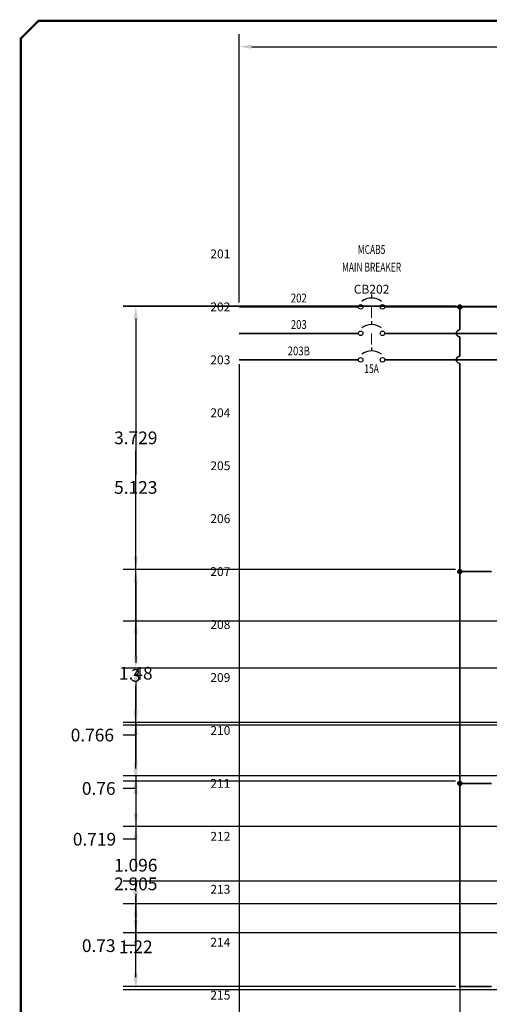
# Model space of a CAD drawing. Extents: x 0 to 33.5, y 0 to 22.4.
# Tile 2 of 8: x 0 to 6.7, y 8.5 to 22.4. Entities that reach past the tile are written whole.
import ezdxf
from ezdxf.enums import TextEntityAlignment as Align

# ---------------------------------------------------------------- set-up
doc = ezdxf.new("R2010")
doc.units = 0
doc.header["$MEASUREMENT"] = 0
for name, color, linetype, lineweight in [('A-ANNO-DIMS', 2, 'Continuous', 18), ('E-ANNO-TEXT', 3, 'Continuous', 18), ('LINK', 9, 'Continuous', 18), ('MISC', 7, 'Continuous', 13), ('SYMS', 7, 'Continuous', 25), ('TITLE', 7, 'Continuous', 35), ('WIRENO', 72, 'Continuous', 18), ('WIRES', 7, 'Continuous', 35)]:
    doc.layers.add(name, color=color, linetype=linetype, lineweight=lineweight)
for name, color, linetype in [('DESC', 150, 'Continuous'), ('TAGS', 150, 'Continuous'), ('XREF', 7, 'Continuous')]:
    doc.layers.add(name, color=color, linetype=linetype)
doc.styles.add('ITALIC', font='ITALIC')
doc.styles.add('SIMPLEX', font='SIMPLEX')
doc.styles.add('WD', font='romans.shx')
doc.dimstyles.get("Standard").update_dxf_attribs({"dimtxt": 0.18, "dimasz": 0.18, "dimexe": 0.18, "dimexo": 0.0625, "dimgap": 0.09, "dimtad": 0, "dimtih": 1, "dimtoh": 1, "dimdec": 4, "dimzin": 0, "dimdsep": 46, "dimtxsty": 'Standard', "dimcen": 0.09, "dimadec": 0, "dimazin": 0, "dimtfac": 1, "dimtdec": 4, "dimtofl": 0, "dimtmove": 0, "dimatfit": 3, "dimfxl": 1, "dimtolj": 1, "dimtzin": 0, "dimarcsym": 0})

# ---------------------------------------------------------------- blocks, each defined once
blk = doc.blocks.new('NO_NUM_acade_title')
at = {"layer": 'TITLE', "const_width": 0.0312}
blk.add_lwpolyline([(30.594, 0.281), (30.594, 22.177), (30.344, 22.427), (0.281, 22.427), (0.031, 22.177), (0.031, 0.281), (0.281, 0.031), (30.344, 0.031)], close=True, dxfattribs=at)
at = {"layer": 'TITLE', "style": 'ITALIC'}
for tag, height, p in [('TITLE#1', 0.125, (32.156, 3.406)), ('TITLE#2', 0.125, (32.156, 3.204)), ('TITLE#3', 0.125, (32.156, 3.001)), ('TITLE#4', 0.125, (32.156, 2.799)), ('DWG#', 0.2, (32.156, 0.826))]:
    blk.add_attdef(tag, text='', height=height, dxfattribs=at).set_placement(p, align=Align.CENTER)
at = {"layer": 'TITLE', "style": 'SIMPLEX'}
blk.add_attdef('CAD#', (30.826, 1.958), '', height=0.0938, rotation=90, dxfattribs=at)
at = {"layer": 'TITLE'}
for tag, p, height, style in [('JOB#', (31.464, 1.644), 0.0938, 'SIMPLEX'), ('SCALE', (31.353, 1.344), 0.0938, 'SIMPLEX'), ('DATE', (32.408, 1.344), 0.0938, 'SIMPLEX'), ('SHTS', (32.532, 0.25), 0.2, 'ITALIC')]:
    blk.add_attdef(tag, p, '', height=height, dxfattribs=dict(at, style=style))
at = {"layer": 'TITLE', "style": 'ITALIC'}
blk.add_attdef('SH#', text='', height=0.2, dxfattribs=at).set_placement((31.881, 0.25), align=Align.RIGHT)
at = {"layer": 'TITLE', "flags": 9}
blk.add_attdef('WD_TB', (31.219, 0.031), '', height=0.125, dxfattribs=at)
blk = doc.blocks.new('WD_MLRH')
at = {"style": 'WD'}
blk.add_attdef('RUNGFIRST', text='', height=0.125, dxfattribs=at).set_placement((-0.25, 0), align=Align.MIDDLE_RIGHT)
at = {"style": 'WD', "flags": 1}
for tag, p in [('RUNGHORV', (-0.25, -0.127)), ('RUNGINC', (-0.25, -0.163)), ('WIREMODE', (-0.25, -0.281)), ('RUNGDIST', (-0.25, -0.2)), ('RUNGCNT', (-0.25, -0.237)), ('WIRE-START', (-0.25, -0.356)), ('WIRE-GSUF', (-0.25, -0.396)), ('PH3SPACE', (-0.25, -0.437)), ('WIREFMT', (-0.25, -0.321))]:
    blk.add_attdef(tag, text='', height=0.025, dxfattribs=at).set_placement(p, align=Align.RIGHT)
blk = doc.blocks.new('HCB1')
blk.add_line((0, 0.173), (0, 0.126))
for centre in [(-0.155, 0), (0.155, 0)]:
    blk.add_circle(centre, 0.0322)
blk.add_arc((0, -0.109), 0.234, 53.1301, 126.8699)
at = {"style": 'WD', "width": 0.7}
for tag, p in [('INST', (0, 0.826)), ('LOC', (0, 0.656)), ('DESC1', (0, 0.5)), ('DESC2', (0, 0.344)), ('RATING1', (0, -0.188)), ('XREF', (0, -0.344))]:
    blk.add_attdef(tag, text='', height=0.125, dxfattribs=at).set_placement(p, align=Align.CENTER)
at = {"style": 'WD'}
blk.add_attdef('TAG1', text='', height=0.125, dxfattribs=at).set_placement((0, 0.188), align=Align.CENTER)
for tag, p in [('X2LINK', (0, 0.219)), ('X8LINK', (0, 0))]:
    blk.add_attdef(tag, p, '', height=0.01, dxfattribs=at)
for tag, p, height, flags in [('CONTACT', (0.205, 0.133), 0.01, 9), ('FAMILY', (0.205, 0.152), 0.01, 9), ('X4TERM01', (-0.188, 0), 0.0125, 1), ('X1TERM02', (0.188, 0), 0.0125, 1)]:
    blk.add_attdef(tag, p, '', height=height, dxfattribs=dict(at, flags=flags))
at = {"style": 'WD', "flags": 9}
for tag, p in [('ASSYCODE', (0.219, 0.062)), ('MFG', (0.228, 0.089)), ('CAT', (0.23, 0.108))]:
    blk.add_attdef(tag, text='', height=0.01, dxfattribs=at).set_placement(p, align=Align.CENTER)
at = {"style": 'WD', "flags": 8}
blk.add_attdef('TERM01', text='', height=0.125, dxfattribs=at).set_placement((-0.25, -0.031), align=Align.TOP_RIGHT)
blk.add_attdef('TERM02', text='', height=0.125, dxfattribs=at).set_placement((0.25, -0.031), align=Align.TOP_LEFT)
blk = doc.blocks.new('WDDOT')
for radius in [0.03, 0.0187, 0.00929]:
    blk.add_circle((0, 0), radius)
blk = doc.blocks.new('WD_WNH')
at = {"style": 'WD', "width": 0.8}
blk.add_attdef('WIRENO', text='', height=0.125, dxfattribs=at).set_placement((0, 0.062), align=Align.CENTER)
at = {"style": 'WD', "flags": 1}
for tag, p in [('W01USER', (0, 0.078)), ('W02USER', (0, 0.07)), ('W03USER', (0, 0.062)), ('W04USER', (0, 0.055)), ('W05USER', (0, 0.047)), ('W06USER', (0, 0.039)), ('W07USER', (0, 0.031)), ('W08USER', (0, 0.023)), ('W09USER', (0, 0.016)), ('W10USER', (0, 0.008))]:
    blk.add_attdef(tag, text='', height=0.005, dxfattribs=at).set_placement(p, align=Align.CENTER)
blk = doc.blocks.new('*D36')
at = {"layer": 'A-ANNO-DIMS', "color": 0, "lineweight": -2, "transparency": 16777216}
for p, q in [((3.125, 17.5625), (3.125, 3.802917)), ((6.25, 17.5625), (6.25, 3.802917)), ((3.305, 3.982917), (4.2675, 3.982917)), ((6.07, 3.982917), (5.1075, 3.982917))]:
    blk.add_line(p, q, dxfattribs=at)
at = {"layer": 'A-ANNO-DIMS', "color": 0, "transparency": 16777216}
for points in [[(3.305, 4.012917), (3.305, 3.952917), (3.125, 3.982917)], [(6.07, 4.012917), (6.07, 3.952917), (6.25, 3.982917)]]:
    blk.add_solid(points, dxfattribs=at)
at = {"layer": 'Defpoints', "color": 0, "transparency": 16777216}
for p in [(3.125, 17.625), (6.25, 17.625), (6.25, 3.982917)]:
    blk.add_point(p, dxfattribs=at)
at = {"layer": 'A-ANNO-DIMS', "color": 0, "transparency": 16777216, "insert": (4.6875, 3.982917), "char_height": 0.18, "attachment_point": 5}
blk.add_mtext('\\A1;3.125', dxfattribs=at)
blk = doc.blocks.new('*D37')
at = {"layer": 'A-ANNO-DIMS', "color": 0, "lineweight": -2, "transparency": 16777216}
for p, q in [((3.125, 18.4375), (3.125, 22.239937)), ((30.05762, 18.46875), (30.05762, 22.239937)), ((3.305, 22.059937), (16.14131, 22.059937)), ((29.87762, 22.059937), (17.04131, 22.059937))]:
    blk.add_line(p, q, dxfattribs=at)
at = {"layer": 'A-ANNO-DIMS', "color": 0, "transparency": 16777216}
for points in [[(3.305, 22.089937), (3.305, 22.029937), (3.125, 22.059937)], [(29.87762, 22.089937), (29.87762, 22.029937), (30.05762, 22.059937)]]:
    blk.add_solid(points, dxfattribs=at)
at = {"layer": 'Defpoints', "color": 0, "transparency": 16777216}
for p in [(30.05762, 22.059937), (3.125, 18.375), (30.05762, 18.40625)]:
    blk.add_point(p, dxfattribs=at)
at = {"layer": 'A-ANNO-DIMS', "color": 0, "transparency": 16777216, "insert": (16.59131, 22.059937), "char_height": 0.18, "attachment_point": 5}
blk.add_mtext('\\A1;26.93', dxfattribs=at)
blk = doc.blocks.new('*D38')
at = {"layer": 'A-ANNO-DIMS', "color": 0, "lineweight": -2, "transparency": 16777216}
for p, q in [((6.188, 18.384), (1.48, 18.384)), ((1.66, 18.204), (1.66, 16.7)), ((1.66, 14.835), (1.66, 16.34)), ((6.188, 14.655), (1.48, 14.655))]:
    blk.add_line(p, q, dxfattribs=at)
at = {"layer": 'A-ANNO-DIMS', "color": 0, "transparency": 16777216}
for points in [[(1.63, 18.204), (1.69, 18.204), (1.66, 18.384)], [(1.63, 14.835), (1.69, 14.835), (1.66, 14.655)]]:
    blk.add_solid(points, dxfattribs=at)
at = {"layer": 'Defpoints', "color": 0, "transparency": 16777216}
for p in [(6.25, 18.384), (1.66, 14.655), (6.25, 14.655)]:
    blk.add_point(p, dxfattribs=at)
at = {"layer": 'A-ANNO-DIMS', "color": 0, "transparency": 16777216, "insert": (1.66, 16.52), "char_height": 0.18, "attachment_point": 5}
blk.add_mtext('\\A1;3.729', dxfattribs=at)
blk = doc.blocks.new('*D39')
at = {"layer": 'A-ANNO-DIMS', "color": 0, "lineweight": -2, "transparency": 16777216}
for p, q in [((6.1875, 14.655), (1.48, 14.655)), ((1.66, 14.475), (1.66, 13.335)), ((1.66, 11.835), (1.66, 12.975)), ((6.1875, 11.655), (1.48, 11.655))]:
    blk.add_line(p, q, dxfattribs=at)
at = {"layer": 'A-ANNO-DIMS', "color": 0, "transparency": 16777216}
for points in [[(1.63, 14.475), (1.69, 14.475), (1.66, 14.655)], [(1.63, 11.835), (1.69, 11.835), (1.66, 11.655)]]:
    blk.add_solid(points, dxfattribs=at)
at = {"layer": 'Defpoints', "color": 0, "transparency": 16777216}
for p in [(6.25, 14.655), (1.66, 11.655), (6.25, 11.655)]:
    blk.add_point(p, dxfattribs=at)
at = {"layer": 'A-ANNO-DIMS', "color": 0, "transparency": 16777216, "insert": (1.66, 13.155), "char_height": 0.18, "attachment_point": 5}
blk.add_mtext('\\A1;3', dxfattribs=at)
blk = doc.blocks.new('*D40')
at = {"layer": 'A-ANNO-DIMS', "color": 0, "lineweight": -2, "transparency": 16777216}
for p, q in [((6.1875, 11.655), (1.48, 11.655)), ((1.66, 11.475), (1.66, 10.3825)), ((1.66, 8.93), (1.66, 10.0225)), ((6.1875, 8.75), (1.48, 8.75))]:
    blk.add_line(p, q, dxfattribs=at)
at = {"layer": 'A-ANNO-DIMS', "color": 0, "transparency": 16777216}
for points in [[(1.63, 11.475), (1.69, 11.475), (1.66, 11.655)], [(1.63, 8.93), (1.69, 8.93), (1.66, 8.75)]]:
    blk.add_solid(points, dxfattribs=at)
at = {"layer": 'Defpoints', "color": 0, "transparency": 16777216}
for p in [(6.25, 11.655), (1.66, 8.75), (6.25, 8.75)]:
    blk.add_point(p, dxfattribs=at)
at = {"layer": 'A-ANNO-DIMS', "color": 0, "transparency": 16777216, "insert": (1.66, 10.2025), "char_height": 0.18, "attachment_point": 5}
blk.add_mtext('\\A1;2.905', dxfattribs=at)
blk = doc.blocks.new('*D46')
at = {"layer": 'A-ANNO-DIMS', "color": 0, "lineweight": -2, "transparency": 16777216}
for p, q in [((13.652, 13.924), (1.48, 13.924)), ((1.66, 13.744), (1.66, 13.366)), ((1.66, 12.628), (1.66, 13.006)), ((13.682, 12.448), (1.48, 12.448))]:
    blk.add_line(p, q, dxfattribs=at)
at = {"layer": 'A-ANNO-DIMS', "color": 0, "transparency": 16777216}
for points in [[(1.63, 13.744), (1.69, 13.744), (1.66, 13.924)], [(1.63, 12.628), (1.69, 12.628), (1.66, 12.448)]]:
    blk.add_solid(points, dxfattribs=at)
at = {"layer": 'Defpoints', "color": 0, "transparency": 16777216}
for p in [(13.715, 13.924), (1.66, 12.448), (13.744, 12.448)]:
    blk.add_point(p, dxfattribs=at)
at = {"layer": 'A-ANNO-DIMS', "color": 0, "transparency": 16777216, "insert": (1.66, 13.186), "char_height": 0.18, "attachment_point": 5}
blk.add_mtext('\\A1;1.48', dxfattribs=at)
blk = doc.blocks.new('*D47')
at = {"layer": 'A-ANNO-DIMS', "color": 0, "lineweight": -2, "transparency": 16777216}
for p, q in [((13.627211, 10.238995), (1.48, 10.238995)), ((1.66, 10.058995), (1.66, 9.686874)), ((13.627211, 9.506874), (1.48, 9.506874)), ((1.66, 9.506874), (1.66, 9.326874)), ((1.66, 9.326874), (1.48, 9.326874))]:
    blk.add_line(p, q, dxfattribs=at)
at = {"layer": 'A-ANNO-DIMS', "color": 0, "transparency": 16777216}
for points in [[(1.63, 10.058995), (1.69, 10.058995), (1.66, 10.238995)], [(1.63, 9.686874), (1.69, 9.686874), (1.66, 9.506874)]]:
    blk.add_solid(points, dxfattribs=at)
at = {"layer": 'Defpoints', "color": 0, "transparency": 16777216}
for p in [(13.689711, 10.238995), (1.66, 9.506874), (13.689711, 9.506874)]:
    blk.add_point(p, dxfattribs=at)
at = {"layer": 'A-ANNO-DIMS', "color": 0, "transparency": 16777216, "insert": (1.135, 9.326874), "char_height": 0.18, "attachment_point": 5}
blk.add_mtext('\\A1;0.73', dxfattribs=at)
blk = doc.blocks.new('*D56')
at = {"layer": 'A-ANNO-DIMS', "color": 0, "lineweight": -2, "transparency": 16777216}
for p, q in [((29.389766, 13.255775), (1.48, 13.255775)), ((1.66, 13.075775), (1.66, 12.669774)), ((29.4322, 12.489774), (1.48, 12.489774)), ((1.66, 12.489774), (1.66, 12.309774)), ((1.66, 12.309774), (1.48, 12.309774))]:
    blk.add_line(p, q, dxfattribs=at)
at = {"layer": 'A-ANNO-DIMS', "color": 0, "transparency": 16777216}
for points in [[(1.63, 13.075775), (1.69, 13.075775), (1.66, 13.255775)], [(1.63, 12.669774), (1.69, 12.669774), (1.66, 12.489774)]]:
    blk.add_solid(points, dxfattribs=at)
at = {"layer": 'Defpoints', "color": 0, "transparency": 16777216}
for p in [(29.452266, 13.255775), (1.66, 12.489774), (29.4947, 12.489774)]:
    blk.add_point(p, dxfattribs=at)
at = {"layer": 'A-ANNO-DIMS', "color": 0, "transparency": 16777216, "insert": (1.045, 12.309774), "char_height": 0.18, "attachment_point": 5}
blk.add_mtext('\\A1;0.766', dxfattribs=at)
blk = doc.blocks.new('*D57')
at = {"layer": 'A-ANNO-DIMS', "color": 0, "lineweight": -2, "transparency": 16777216}
for p, q in [((29.4322, 12.489774), (1.48, 12.489774)), ((1.66, 12.309774), (1.66, 11.913516)), ((29.435818, 11.733516), (1.48, 11.733516)), ((1.66, 11.733516), (1.66, 11.553516)), ((1.66, 11.553516), (1.48, 11.553516))]:
    blk.add_line(p, q, dxfattribs=at)
at = {"layer": 'A-ANNO-DIMS', "color": 0, "transparency": 16777216}
for points in [[(1.63, 12.309774), (1.69, 12.309774), (1.66, 12.489774)], [(1.63, 11.913516), (1.69, 11.913516), (1.66, 11.733516)]]:
    blk.add_solid(points, dxfattribs=at)
at = {"layer": 'Defpoints', "color": 0, "transparency": 16777216}
for p in [(29.4947, 12.489774), (1.66, 11.733516), (29.498318, 11.733516)]:
    blk.add_point(p, dxfattribs=at)
at = {"layer": 'A-ANNO-DIMS', "color": 0, "transparency": 16777216, "insert": (1.135, 11.553516), "char_height": 0.18, "attachment_point": 5}
blk.add_mtext('\\A1;0.76', dxfattribs=at)
blk = doc.blocks.new('*D58')
at = {"layer": 'A-ANNO-DIMS', "color": 0, "lineweight": -2, "transparency": 16777216}
for p, q in [((29.435818, 11.733516), (1.48, 11.733516)), ((1.66, 11.553516), (1.66, 11.194575)), ((29.438773, 11.014575), (1.48, 11.014575)), ((1.66, 11.014575), (1.66, 10.834575)), ((1.66, 10.834575), (1.48, 10.834575))]:
    blk.add_line(p, q, dxfattribs=at)
at = {"layer": 'A-ANNO-DIMS', "color": 0, "transparency": 16777216}
for points in [[(1.63, 11.553516), (1.69, 11.553516), (1.66, 11.733516)], [(1.63, 11.194575), (1.69, 11.194575), (1.66, 11.014575)]]:
    blk.add_solid(points, dxfattribs=at)
at = {"layer": 'Defpoints', "color": 0, "transparency": 16777216}
for p in [(29.498318, 11.733516), (1.66, 11.014575), (29.501273, 11.014575)]:
    blk.add_point(p, dxfattribs=at)
at = {"layer": 'A-ANNO-DIMS', "color": 0, "transparency": 16777216, "insert": (1.075, 10.834575), "char_height": 0.18, "attachment_point": 5}
blk.add_mtext('\\A1;0.719', dxfattribs=at)
blk = doc.blocks.new('*D59')
at = {"layer": 'A-ANNO-DIMS', "color": 0, "lineweight": -2, "transparency": 16777216}
for p, q in [((29.438773, 11.014575), (1.48, 11.014575)), ((1.66, 10.834575), (1.66, 10.646575)), ((1.66, 10.098575), (1.66, 10.286575)), ((29.435818, 9.918575), (1.48, 9.918575))]:
    blk.add_line(p, q, dxfattribs=at)
at = {"layer": 'A-ANNO-DIMS', "color": 0, "transparency": 16777216}
for points in [[(1.63, 10.834575), (1.69, 10.834575), (1.66, 11.014575)], [(1.63, 10.098575), (1.69, 10.098575), (1.66, 9.918575)]]:
    blk.add_solid(points, dxfattribs=at)
at = {"layer": 'Defpoints', "color": 0, "transparency": 16777216}
for p in [(29.501273, 11.014575), (1.66, 9.918575), (29.498318, 9.918575)]:
    blk.add_point(p, dxfattribs=at)
at = {"layer": 'A-ANNO-DIMS', "color": 0, "transparency": 16777216, "insert": (1.66, 10.466575), "char_height": 0.18, "attachment_point": 5}
blk.add_mtext('\\A1;1.096', dxfattribs=at)
blk = doc.blocks.new('*D60')
at = {"layer": 'A-ANNO-DIMS', "color": 0, "lineweight": -2, "transparency": 16777216}
for p, q in [((29.435818, 9.918575), (1.48, 9.918575)), ((1.66, 9.738575), (1.66, 9.490438)), ((1.66, 8.882301), (1.66, 9.130438)), ((29.4322, 8.702301), (1.48, 8.702301))]:
    blk.add_line(p, q, dxfattribs=at)
at = {"layer": 'A-ANNO-DIMS', "color": 0, "transparency": 16777216}
for points in [[(1.63, 9.738575), (1.69, 9.738575), (1.66, 9.918575)], [(1.63, 8.882301), (1.69, 8.882301), (1.66, 8.702301)]]:
    blk.add_solid(points, dxfattribs=at)
at = {"layer": 'Defpoints', "color": 0, "transparency": 16777216}
for p in [(29.498318, 9.918575), (1.66, 8.702301), (29.4947, 8.702301)]:
    blk.add_point(p, dxfattribs=at)
at = {"layer": 'A-ANNO-DIMS', "color": 0, "transparency": 16777216, "insert": (1.66, 9.310438), "char_height": 0.18, "attachment_point": 5}
blk.add_mtext('\\A1;1.22', dxfattribs=at)
blk = doc.blocks.new('*D61')
at = {"layer": 'A-ANNO-DIMS', "color": 0, "lineweight": -2, "transparency": 16777216}
for p, q in [((23.088, 18.379), (1.48, 18.379)), ((1.66, 18.199), (1.66, 15.997)), ((1.66, 13.436), (1.66, 15.637)), ((20.838, 13.256), (1.48, 13.256))]:
    blk.add_line(p, q, dxfattribs=at)
at = {"layer": 'A-ANNO-DIMS', "color": 0, "transparency": 16777216}
for points in [[(1.63, 18.199), (1.69, 18.199), (1.66, 18.379)], [(1.63, 13.436), (1.69, 13.436), (1.66, 13.256)]]:
    blk.add_solid(points, dxfattribs=at)
at = {"layer": 'Defpoints', "color": 0, "transparency": 16777216}
for p in [(23.151, 18.379), (1.66, 13.256), (20.901, 13.256)]:
    blk.add_point(p, dxfattribs=at)
at = {"layer": 'A-ANNO-DIMS', "color": 0, "transparency": 16777216, "insert": (1.66, 15.817), "char_height": 0.18, "attachment_point": 5}
blk.add_mtext('\\A1;5.123', dxfattribs=at)

msp = doc.modelspace()

# ---------------------------------------------------------------- linework, layer by layer
at = {"layer": 'LINK'}
for points in [[(5, 18.375), (5, 18.2188)], [(5, 18), (5, 17.8438)]]:
    msp.add_lwpolyline(points, dxfattribs=at)
at = {"layer": 'WIRES'}
for p, q in [((3.125, 18.375), (4.8125, 18.375)), ((5.1875, 18.375), (30.0576, 18.375)), ((6.25, 18.375), (6.25, 18.05)), ((3.125, 18), (4.8125, 18)), ((5.1875, 18), (30.0939, 18)), ((6.25, 17.95), (6.25, 17.675)), ((3.125, 17.625), (4.8125, 17.625)), ((5.1875, 17.625), (30.0939, 17.625)), ((6.25, 17.575), (6.25, 8.75)), ((6.25, 14.625), (6.7, 14.625)), ((6.25, 11.625), (6.7, 11.625)), ((6.25, 8.75), (6.7, 8.75))]:
    msp.add_line(p, q, dxfattribs=at)
for centre in [(6.25, 18), (6.25, 17.625)]:
    msp.add_arc(centre, 0.05, 90, 270, dxfattribs=at)

# ---------------------------------------------------------------- block references
at = {"layer": 'MISC'}
msp.add_blockref('WD_MLRH', (3.25, 19.125), dxfattribs=at).add_auto_attribs({'RUNGFIRST': '201'})
at = {"layer": 'SYMS'}
ref = msp.add_blockref('HCB1', (5, 18.375), dxfattribs=at)
ref.add_attrib('XREF', 'MCAB5', dxfattribs={"layer": 'XREF', "height": 0.125, "style": 'WD', "width": 0.7}).set_placement((5, 19.125), align=Align.CENTER)
ref.add_attrib('DESC1', 'MAIN BREAKER', dxfattribs={"layer": 'DESC', "height": 0.125, "style": 'WD', "width": 0.7}).set_placement((5, 18.875), align=Align.CENTER)
ref.add_attrib('TAG1', 'CB202', dxfattribs={"layer": 'TAGS', "height": 0.125, "style": 'WD'}).set_placement((5, 18.5625), align=Align.CENTER)
for name, p in [('WDDOT', (6.25, 18.375)), ('HCB1', (5, 18)), ('WDDOT', (6.25, 14.625)), ('WDDOT', (6.25, 11.625))]:
    msp.add_blockref(name, p, dxfattribs=at)
ref = msp.add_blockref('HCB1', (5, 17.625), dxfattribs=at)
ref.add_attrib('RATING1', '15A', dxfattribs={"layer": 'MISC', "height": 0.125, "style": 'WD', "width": 0.7}).set_placement((5, 17.4375), align=Align.CENTER)
at = {"layer": 'TITLE'}
msp.add_blockref('NO_NUM_acade_title', (0, 0), dxfattribs=at)
at = {"layer": 'WIRENO'}
ref = msp.add_blockref('WD_WNH', (3.9688, 18.375), dxfattribs=at)
ref.add_attrib('WIRENO', '202', dxfattribs={"linetype": 'Continuous', "height": 0.125, "style": 'WD', "width": 0.8}).set_placement((3.9688, 18.4375), align=Align.CENTER)
ref = msp.add_blockref('WD_WNH', (3.9688, 18), dxfattribs=at)
ref.add_attrib('WIRENO', '203', dxfattribs={"linetype": 'Continuous', "height": 0.125, "style": 'WD', "width": 0.8}).set_placement((3.9688, 18.0625), align=Align.CENTER)
ref = msp.add_blockref('WD_WNH', (3.9688, 17.625), dxfattribs=at)
ref.add_attrib('WIRENO', '203B', dxfattribs={"linetype": 'Continuous', "height": 0.125, "style": 'WD', "width": 0.8}).set_placement((3.9688, 17.6875), align=Align.CENTER)

# ---------------------------------------------------------------- texts
at = {"layer": 'E-ANNO-TEXT', "style": 'WD'}
for s, p in [('202', (3, 18.375)), ('203', (3, 17.625)), ('204', (3, 16.875)), ('205', (3, 16.125)), ('206', (3, 15.375)), ('207', (3, 14.625)), ('208', (3, 13.875)), ('209', (3, 13.125)), ('210', (3, 12.375)), ('211', (3, 11.625)), ('212', (3, 10.875)), ('213', (3, 10.125)), ('214', (3, 9.375)), ('215', (3, 8.625))]:
    msp.add_text(s, height=0.125, dxfattribs=at).set_placement(p, align=Align.MIDDLE_RIGHT)

# ---------------------------------------------------------------- dimensions: what is measured, and where the dimension line sits
at = {"layer": 'A-ANNO-DIMS'}
for base, p1, p2, override, picture, middle in [((30.0576, 22.0599), (3.125, 18.375), (30.0576, 18.4062), {"dimdec": 2, "dimlfac": 1, "dimrnd": 0, "dimzin": 0, "dimdsep": 46, "dimlunit": 2}, '*D37', (16.5913, 22.0599)), ((6.25, 3.9829), (3.125, 17.625), (6.25, 17.625), {"dimdec": 3, "dimlfac": 1, "dimrnd": 0, "dimzin": 0, "dimdsep": 46, "dimlunit": 2}, '*D36', (4.6875, 3.9829))]:
    dim = msp.add_linear_dim(base=base, p1=p1, p2=p2, dimstyle='Standard', override=override, dxfattribs=at)
    dim.commit()
    dim.dimension.update_dxf_attribs({"geometry": picture, "text_midpoint": middle})
for base, p1, p2, override, picture, middle in [((1.66, 14.655), (6.25, 18.3843), (6.25, 14.655), {"dimdec": 3, "dimlfac": 1, "dimrnd": 0, "dimzin": 0, "dimdsep": 46, "dimlunit": 2}, '*D38', (1.66, 16.5196)), ((1.66, 13.2558), (23.151, 18.3786), (20.9008, 13.2558), {"dimdec": 3, "dimlfac": 1, "dimrnd": 0, "dimzin": 0, "dimdsep": 46, "dimlunit": 2}, '*D61', (1.66, 15.8172)), ((1.66, 11.655), (6.25, 14.655), (6.25, 11.655), {"dimdec": 0, "dimlfac": 1, "dimrnd": 0, "dimzin": 0, "dimdsep": 46, "dimlunit": 2}, '*D39', (1.66, 13.155)), ((1.66, 12.448), (13.7148, 13.9244), (13.7441, 12.448), {"dimdec": 2, "dimlfac": 1, "dimrnd": 0, "dimzin": 0, "dimdsep": 46, "dimlunit": 2}, '*D46', (1.66, 13.1862)), ((1.66, 12.4898), (29.4523, 13.2558), (29.4947, 12.4898), {"dimdec": 3, "dimlfac": 1, "dimrnd": 0, "dimzin": 0, "dimdsep": 46, "dimlunit": 2}, '*D56', (1.045, 12.3098)), ((1.66, 11.7335), (29.4947, 12.4898), (29.4983, 11.7335), {"dimdec": 2, "dimlfac": 1, "dimrnd": 0, "dimzin": 0, "dimdsep": 46, "dimlunit": 2}, '*D57', (1.135, 11.5535)), ((1.66, 11.0146), (29.4983, 11.7335), (29.5013, 11.0146), {"dimdec": 3, "dimlfac": 1, "dimrnd": 0, "dimzin": 0, "dimdsep": 46, "dimlunit": 2}, '*D58', (1.075, 10.8346)), ((1.66, 8.75), (6.25, 11.655), (6.25, 8.75), {"dimdec": 3, "dimlfac": 1, "dimrnd": 0, "dimzin": 0, "dimdsep": 46, "dimlunit": 2}, '*D40', (1.66, 10.2025)), ((1.66, 9.9186), (29.5013, 11.0146), (29.4983, 9.9186), {"dimdec": 3, "dimlfac": 1, "dimrnd": 0, "dimzin": 0, "dimdsep": 46, "dimlunit": 2}, '*D59', (1.66, 10.4666)), ((1.66, 9.5069), (13.6897, 10.239), (13.6897, 9.5069), {"dimdec": 2, "dimlfac": 1, "dimrnd": 0, "dimzin": 0, "dimdsep": 46, "dimlunit": 2}, '*D47', (1.135, 9.3269)), ((1.66, 8.7023), (29.4983, 9.9186), (29.4947, 8.7023), {"dimdec": 2, "dimlfac": 1, "dimrnd": 0, "dimzin": 0, "dimdsep": 46, "dimlunit": 2}, '*D60', (1.66, 9.3104))]:
    dim = msp.add_linear_dim(base=base, p1=p1, p2=p2, angle=90, dimstyle='Standard', override=override, dxfattribs=at)
    dim.commit()
    dim.dimension.update_dxf_attribs({"geometry": picture, "text_midpoint": middle})

doc.saveas('drawing.dxf')
